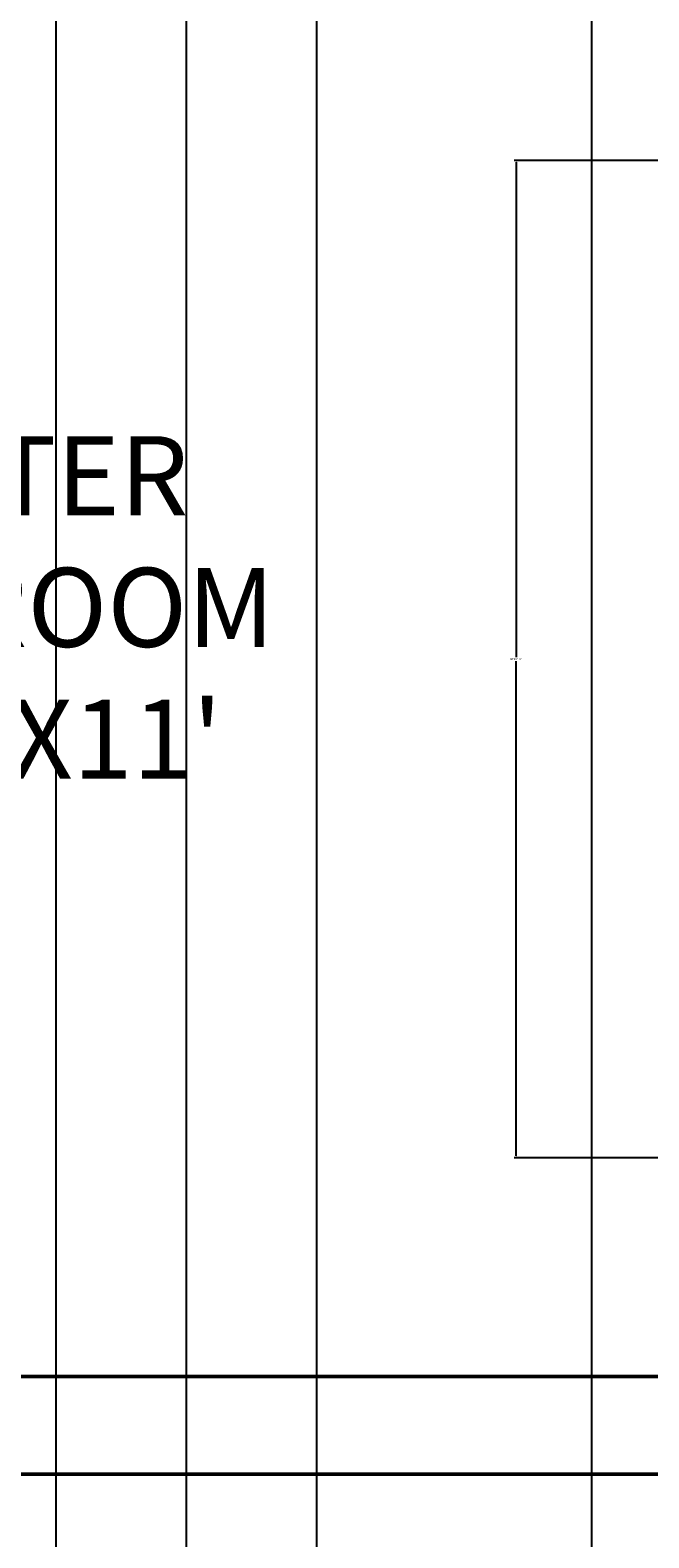
# Model space of a CAD drawing. Units: inches. Extents: x 338 to 1188, y -996 to 127.
# Tile 9 of 15: x 802 to 859, y -622 to -483. Entities that reach past the tile are written whole.
import ezdxf

# ---------------------------------------------------------------- set-up
doc = ezdxf.new("R2010")
doc.units = ezdxf.units.IN
doc.header["$MEASUREMENT"] = 0
for name, color, linetype, lineweight in [('A-ANNO-DIMS', 5, 'Continuous', 18), ('A-AREA-IDEN', 8, 'Continuous', 18), ('wall', 1, 'Continuous', 50)]:
    doc.layers.add(name, color=color, linetype=linetype, lineweight=lineweight)
doc.styles.get("Standard").update_dxf_attribs({"font": 'arial.ttf'})
doc.dimstyles.get("Standard").update_dxf_attribs({"dimtxt": 0.18, "dimasz": 0.18, "dimexe": 0.18, "dimexo": 0.0625, "dimgap": 0.09, "dimtad": 0, "dimtih": 1, "dimtoh": 1, "dimdec": 1, "dimzin": 0, "dimdsep": 46, "dimlunit": 4, "dimtxsty": 'Standard', "dimcen": 0.09, "dimadec": 0, "dimazin": 0, "dimtfac": 1, "dimtdec": 1, "dimtofl": 0, "dimtmove": 0, "dimatfit": 3, "dimfxl": 1, "dimtolj": 1, "dimtzin": 0, "dimarcsym": 0})

# ---------------------------------------------------------------- blocks, each defined once
blk = doc.blocks.new('*D19')
at = {"layer": 'A-ANNO-DIMS', "color": 0, "lineweight": -2, "transparency": 16777216}
for p, q in [((860.06, -494.84), (846.17, -494.84)), ((846.35, -495.02), (846.35, -540.55)), ((846.35, -586.45), (846.35, -540.91)), ((860.06, -586.63), (846.17, -586.63))]:
    blk.add_line(p, q, dxfattribs=at)
at = {"layer": 'A-ANNO-DIMS', "color": 0, "transparency": 16777216}
for points in [[(846.32, -495.02), (846.38, -495.02), (846.35, -494.84)], [(846.32, -586.45), (846.38, -586.45), (846.35, -586.63)]]:
    blk.add_solid(points, dxfattribs=at)
at = {"layer": 'Defpoints', "color": 0, "transparency": 16777216}
for p in [(860.12, -494.84), (846.35, -586.63), (860.12, -586.63)]:
    blk.add_point(p, dxfattribs=at)
at = {"layer": 'A-ANNO-DIMS', "color": 0, "transparency": 16777216, "insert": (846.35, -540.73), "char_height": 0.18, "attachment_point": 5}
blk.add_mtext('\\A1;BED 7\'-8"', dxfattribs=at)
blk = doc.blocks.new('*D26')
at = {"layer": 'A-ANNO-DIMS', "color": 0, "lineweight": -2, "transparency": 16777216}
for p, q in [((815.96, -297.8), (815.96, -968.86)), ((827.96, -297.8), (827.96, -968.86)), ((816.14, -968.68), (821.64, -968.68)), ((827.78, -968.68), (822.28, -968.68))]:
    blk.add_line(p, q, dxfattribs=at)
at = {"layer": 'A-ANNO-DIMS', "color": 0, "transparency": 16777216}
for points in [[(816.14, -968.65), (816.14, -968.71), (815.96, -968.68)], [(827.78, -968.65), (827.78, -968.71), (827.96, -968.68)]]:
    blk.add_solid(points, dxfattribs=at)
at = {"layer": 'Defpoints', "color": 0, "transparency": 16777216}
for p in [(815.96, -297.73), (827.96, -297.73), (827.96, -968.68)]:
    blk.add_point(p, dxfattribs=at)
at = {"layer": 'A-ANNO-DIMS', "color": 0, "transparency": 16777216, "insert": (821.96, -968.68), "char_height": 0.18, "attachment_point": 5}
blk.add_mtext('\\A1;1\'-0"', dxfattribs=at)
blk = doc.blocks.new('*D28')
at = {"layer": 'A-ANNO-DIMS', "color": 0, "lineweight": -2, "transparency": 16777216}
for p, q in [((803.96, -265.8), (803.96, -968.86)), ((947.96, -297.8), (947.96, -968.86)), ((804.14, -968.68), (875.57, -968.68)), ((947.78, -968.68), (876.35, -968.68))]:
    blk.add_line(p, q, dxfattribs=at)
at = {"layer": 'A-ANNO-DIMS', "color": 0, "transparency": 16777216}
for points in [[(804.14, -968.65), (804.14, -968.71), (803.96, -968.68)], [(947.78, -968.65), (947.78, -968.71), (947.96, -968.68)]]:
    blk.add_solid(points, dxfattribs=at)
at = {"layer": 'Defpoints', "color": 0, "transparency": 16777216}
for p in [(803.96, -265.73), (947.96, -297.73), (947.96, -968.68)]:
    blk.add_point(p, dxfattribs=at)
at = {"layer": 'A-ANNO-DIMS', "color": 0, "transparency": 16777216, "insert": (875.96, -968.68), "char_height": 0.18, "attachment_point": 5}
blk.add_mtext('\\A1;12\'-0"', dxfattribs=at)
blk = doc.blocks.new('*D43')
at = {"layer": 'A-ANNO-DIMS', "color": 0, "lineweight": -2, "transparency": 16777216}
for p, q in [((853.28, -53.93), (853.28, -968.86)), ((895.37, -53.93), (895.37, -968.86)), ((853.46, -968.68), (873.99, -968.68)), ((895.19, -968.68), (874.65, -968.68))]:
    blk.add_line(p, q, dxfattribs=at)
at = {"layer": 'A-ANNO-DIMS', "color": 0, "transparency": 16777216}
for points in [[(853.46, -968.65), (853.46, -968.71), (853.28, -968.68)], [(895.19, -968.65), (895.19, -968.71), (895.37, -968.68)]]:
    blk.add_solid(points, dxfattribs=at)
at = {"layer": 'Defpoints', "color": 0, "transparency": 16777216}
for p in [(853.28, -53.87), (895.37, -53.87), (895.37, -968.68)]:
    blk.add_point(p, dxfattribs=at)
at = {"layer": 'A-ANNO-DIMS', "color": 0, "transparency": 16777216, "insert": (874.32, -968.68), "char_height": 0.18, "attachment_point": 5}
blk.add_mtext('\\A1;3\'-6"', dxfattribs=at)
blk = doc.blocks.new('*D47')
at = {"layer": 'A-ANNO-DIMS', "color": 0, "lineweight": -2, "transparency": 16777216}
for p, q in [((759.67, -755.17), (759.67, 67.25)), ((759.85, 67.07), (867.68, 67.07)), ((976.28, 67.07), (868.46, 67.07)), ((976.46, -755.17), (976.46, 67.25))]:
    blk.add_line(p, q, dxfattribs=at)
at = {"layer": 'A-ANNO-DIMS', "color": 0, "transparency": 16777216}
for points in [[(759.85, 67.1), (759.85, 67.04), (759.67, 67.07)], [(976.28, 67.1), (976.28, 67.04), (976.46, 67.07)]]:
    blk.add_solid(points, dxfattribs=at)
at = {"layer": 'Defpoints', "color": 0, "transparency": 16777216}
for p in [(976.46, 67.07), (759.67, -755.23), (976.46, -755.23)]:
    blk.add_point(p, dxfattribs=at)
at = {"layer": 'A-ANNO-DIMS', "color": 0, "transparency": 16777216, "insert": (868.07, 67.07), "char_height": 0.18, "attachment_point": 5}
blk.add_mtext('\\A1;18\'-1"', dxfattribs=at)

msp = doc.modelspace()

# ---------------------------------------------------------------- linework, layer by layer
at = {"layer": 'wall'}
for p, q in [((947.96, -606.73), (746.96, -606.73)), ((956.96, -615.73), (660.96, -615.73))]:
    msp.add_line(p, q, dxfattribs=at)

# ---------------------------------------------------------------- texts
at = {"layer": 'A-AREA-IDEN', "insert": (775.86, -520.22), "char_height": 7.2703, "attachment_point": 1}
msp.add_mtext_dynamic_manual_height_columns(' MASTER   BEDROOM              16\'9"X11\'', width=58.3567, gutter_width=1, heights=[0], dxfattribs=at)

# ---------------------------------------------------------------- dimensions: what is measured, and where the dimension line sits
at = {"layer": 'A-ANNO-DIMS'}
for base, p1, p2, picture, middle in [((976.46, 67.07), (759.67, -755.23), (976.46, -755.23), '*D47', (868.07, 67.07)), ((895.37, -968.68), (853.28, -53.87), (895.37, -53.87), '*D43', (874.32, -968.68)), ((947.96, -968.68), (803.96, -265.73), (947.96, -297.73), '*D28', (875.96, -968.68)), ((827.96, -968.68), (815.96, -297.73), (827.96, -297.73), '*D26', (821.96, -968.68))]:
    dim = msp.add_linear_dim(base=base, p1=p1, p2=p2, dimstyle='Standard', override={"dimdec": 1, "dimlfac": 1, "dimrnd": 0, "dimzin": 1, "dimdsep": 46, "dimlunit": 4, "dimfrac": 2}, dxfattribs=at)
    dim.commit()
    dim.dimension.update_dxf_attribs({"geometry": picture, "text_midpoint": middle})
dim = msp.add_linear_dim(base=(846.35, -586.63), p1=(860.12, -494.84), p2=(860.12, -586.63), angle=270, text='BED <>', dimstyle='Standard', override={"dimdec": 1, "dimlfac": 1, "dimrnd": 0, "dimzin": 1, "dimdsep": 46, "dimlunit": 4, "dimfrac": 2}, dxfattribs=at)
dim.commit()
dim.dimension.update_dxf_attribs({"geometry": '*D19', "text_midpoint": (846.35, -540.73)})

doc.saveas('drawing.dxf')
